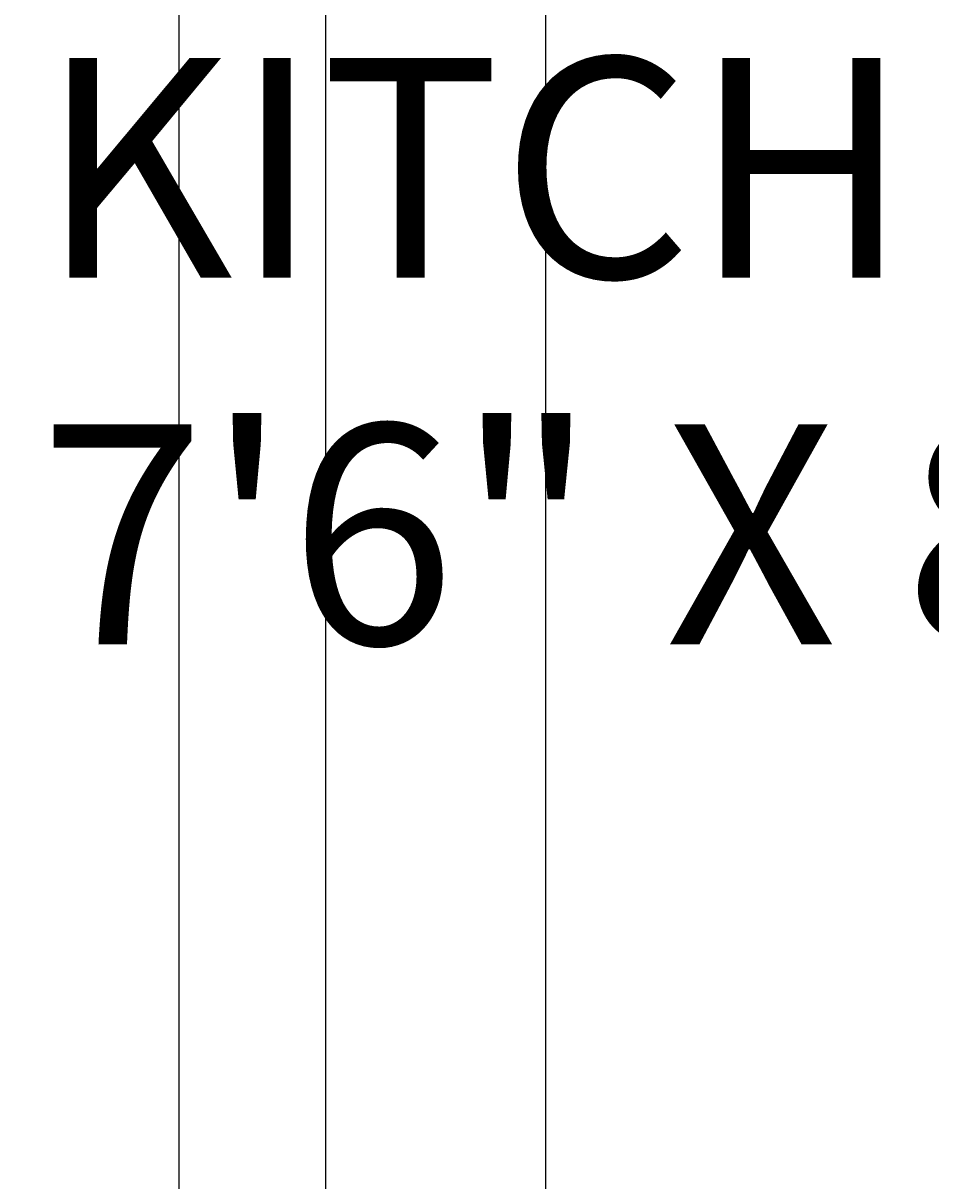
# Model space of a CAD drawing. Units: inches. Extents: x 37 to 824, y -700 to 234.
# Tile 31 of 77: x 202 to 227, y -237 to -206. Entities that reach past the tile are written whole.
import ezdxf

# ---------------------------------------------------------------- set-up
doc = ezdxf.new("R2010")
doc.units = ezdxf.units.IN
doc.header["$MEASUREMENT"] = 0
doc.layers.add('A-ANNO-DIMS', color=2, linetype='Continuous', lineweight=18)
doc.layers.add('A-AREA-IDEN', color=3, linetype='Continuous', lineweight=18)
doc.styles.get("Standard").update_dxf_attribs({"font": 'arial.ttf'})
doc.dimstyles.get("Standard").update_dxf_attribs({"dimtxt": 0.18, "dimasz": 0.18, "dimexe": 0.18, "dimexo": 0.0625, "dimgap": 0.09, "dimtad": 0, "dimtih": 1, "dimtoh": 1, "dimdec": 1, "dimzin": 0, "dimdsep": 46, "dimlunit": 4, "dimtxsty": 'Standard', "dimcen": 0.09, "dimadec": 0, "dimazin": 0, "dimtfac": 1, "dimtdec": 1, "dimtofl": 0, "dimtmove": 0, "dimatfit": 3, "dimfxl": 1, "dimtolj": 1, "dimtzin": 0, "dimarcsym": 0})

# ---------------------------------------------------------------- blocks, each defined once
blk = doc.blocks.new('*D80')
at = {"layer": 'A-ANNO-DIMS', "color": 0, "lineweight": -2, "ltscale": 0.5, "transparency": 16777216}
for p, q in [((170.077, -167.972), (170.077, -400.406)), ((250.19, -167.972), (250.19, -400.406)), ((170.257, -400.226), (209.804, -400.226)), ((250.01, -400.226), (210.463, -400.226))]:
    blk.add_line(p, q, dxfattribs=at)
at = {"layer": 'A-ANNO-DIMS', "color": 0, "ltscale": 0.5, "transparency": 16777216}
for points in [[(170.257, -400.196), (170.257, -400.256), (170.077, -400.226)], [(250.01, -400.196), (250.01, -400.256), (250.19, -400.226)]]:
    blk.add_solid(points, dxfattribs=at)
at = {"layer": 'Defpoints', "color": 0, "ltscale": 0.5, "transparency": 16777216}
for p in [(170.077, -167.91), (250.19, -167.91), (250.19, -400.226)]:
    blk.add_point(p, dxfattribs=at)
at = {"layer": 'A-ANNO-DIMS', "color": 0, "ltscale": 0.5, "transparency": 16777216, "insert": (210.133, -400.226), "char_height": 0.18, "attachment_point": 5}
blk.add_mtext('\\A1;6\'-8"', dxfattribs=at)
blk = doc.blocks.new('*D84')
at = {"layer": 'A-ANNO-DIMS', "color": 0, "lineweight": -2, "ltscale": 0.5, "transparency": 16777216}
for p, q in [((170.077, -265.847), (170.077, 234.17)), ((210.077, -265.847), (210.077, 234.17)), ((170.257, 233.99), (189.748, 233.99)), ((209.897, 233.99), (190.406, 233.99))]:
    blk.add_line(p, q, dxfattribs=at)
at = {"layer": 'A-ANNO-DIMS', "color": 0, "ltscale": 0.5, "transparency": 16777216}
for points in [[(170.257, 234.02), (170.257, 233.96), (170.077, 233.99)], [(209.897, 234.02), (209.897, 233.96), (210.077, 233.99)]]:
    blk.add_solid(points, dxfattribs=at)
at = {"layer": 'Defpoints', "color": 0, "ltscale": 0.5, "transparency": 16777216}
for p in [(210.077, 233.99), (170.077, -265.91), (210.077, -265.91)]:
    blk.add_point(p, dxfattribs=at)
at = {"layer": 'A-ANNO-DIMS', "color": 0, "ltscale": 0.5, "transparency": 16777216, "insert": (190.077, 233.99), "char_height": 0.18, "attachment_point": 5}
blk.add_mtext('\\A1;3\'-4"', dxfattribs=at)
blk = doc.blocks.new('*D85')
at = {"layer": 'A-ANNO-DIMS', "color": 0, "lineweight": -2, "ltscale": 0.5, "transparency": 16777216}
for p, q in [((170.077, -356.847), (170.077, 234.17)), ((206.077, -356.847), (206.077, 234.17)), ((170.257, 233.99), (187.748, 233.99)), ((205.897, 233.99), (188.406, 233.99))]:
    blk.add_line(p, q, dxfattribs=at)
at = {"layer": 'A-ANNO-DIMS', "color": 0, "ltscale": 0.5, "transparency": 16777216}
for points in [[(170.257, 234.02), (170.257, 233.96), (170.077, 233.99)], [(205.897, 234.02), (205.897, 233.96), (206.077, 233.99)]]:
    blk.add_solid(points, dxfattribs=at)
at = {"layer": 'Defpoints', "color": 0, "ltscale": 0.5, "transparency": 16777216}
for p in [(206.077, 233.99), (170.077, -356.91), (206.077, -356.91)]:
    blk.add_point(p, dxfattribs=at)
at = {"layer": 'A-ANNO-DIMS', "color": 0, "ltscale": 0.5, "transparency": 16777216, "insert": (188.077, 233.99), "char_height": 0.18, "attachment_point": 5}
blk.add_mtext('\\A1;3\'-0"', dxfattribs=at)
blk = doc.blocks.new('*D86')
at = {"layer": 'A-ANNO-DIMS', "color": 0, "lineweight": -2, "ltscale": 0.5, "transparency": 16777216}
for p, q in [((206.077, -356.847), (206.077, 234.17)), ((216.077, -356.847), (216.077, 234.17)), ((206.257, 233.99), (210.678, 233.99)), ((215.897, 233.99), (211.476, 233.99))]:
    blk.add_line(p, q, dxfattribs=at)
at = {"layer": 'A-ANNO-DIMS', "color": 0, "ltscale": 0.5, "transparency": 16777216}
for points in [[(206.257, 234.02), (206.257, 233.96), (206.077, 233.99)], [(215.897, 234.02), (215.897, 233.96), (216.077, 233.99)]]:
    blk.add_solid(points, dxfattribs=at)
at = {"layer": 'Defpoints', "color": 0, "ltscale": 0.5, "transparency": 16777216}
for p in [(216.077, 233.99), (206.077, -356.91), (216.077, -356.91)]:
    blk.add_point(p, dxfattribs=at)
at = {"layer": 'A-ANNO-DIMS', "color": 0, "ltscale": 0.5, "transparency": 16777216, "insert": (211.077, 233.99), "char_height": 0.18, "attachment_point": 5}
blk.add_mtext('\\A1;0\'-10"', dxfattribs=at)
blk = doc.blocks.new('*D87')
at = {"layer": 'A-ANNO-DIMS', "color": 0, "lineweight": -2, "ltscale": 0.5, "transparency": 16777216}
for p, q in [((216.077, -356.847), (216.077, 234.17)), ((296.077, -356.847), (296.077, 234.17)), ((216.257, 233.99), (255.747, 233.99)), ((295.897, 233.99), (256.407, 233.99))]:
    blk.add_line(p, q, dxfattribs=at)
at = {"layer": 'A-ANNO-DIMS', "color": 0, "ltscale": 0.5, "transparency": 16777216}
for points in [[(216.257, 234.02), (216.257, 233.96), (216.077, 233.99)], [(295.897, 234.02), (295.897, 233.96), (296.077, 233.99)]]:
    blk.add_solid(points, dxfattribs=at)
at = {"layer": 'Defpoints', "color": 0, "ltscale": 0.5, "transparency": 16777216}
for p in [(296.077, 233.99), (216.077, -356.91), (296.077, -356.91)]:
    blk.add_point(p, dxfattribs=at)
at = {"layer": 'A-ANNO-DIMS', "color": 0, "ltscale": 0.5, "transparency": 16777216, "insert": (256.077, 233.99), "char_height": 0.18, "attachment_point": 5}
blk.add_mtext('\\A1;6\'-8"', dxfattribs=at)

msp = doc.modelspace()

# ---------------------------------------------------------------- texts
at = {"layer": 'A-AREA-IDEN', "insert": (202.252, -206.696), "char_height": 6, "attachment_point": 1}
msp.add_mtext_dynamic_manual_height_columns('KITCHEN\\P7\'6" X 8\'2"', width=88.32168, gutter_width=1, heights=[0], dxfattribs=at)

# ---------------------------------------------------------------- dimensions: what is measured, and where the dimension line sits
at = {"layer": 'A-ANNO-DIMS', "ltscale": 0.5}
for base, p1, p2, picture, middle in [((210.077, 233.99), (170.077, -265.91), (210.077, -265.91), '*D84', (190.077, 233.99)), ((206.077, 233.99), (170.077, -356.91), (206.077, -356.91), '*D85', (188.077, 233.99)), ((216.077, 233.99), (206.077, -356.91), (216.077, -356.91), '*D86', (211.077, 233.99)), ((296.077, 233.99), (216.077, -356.91), (296.077, -356.91), '*D87', (256.077, 233.99)), ((250.19, -400.226), (170.077, -167.91), (250.19, -167.91), '*D80', (210.133, -400.226))]:
    dim = msp.add_linear_dim(base=base, p1=p1, p2=p2, dimstyle='Standard', override={"dimdec": 1, "dimlfac": 1, "dimrnd": 0, "dimzin": 1, "dimdsep": 46, "dimlunit": 4, "dimfrac": 2}, dxfattribs=at)
    dim.commit()
    dim.dimension.update_dxf_attribs({"geometry": picture, "text_midpoint": middle})

doc.saveas('drawing.dxf')
